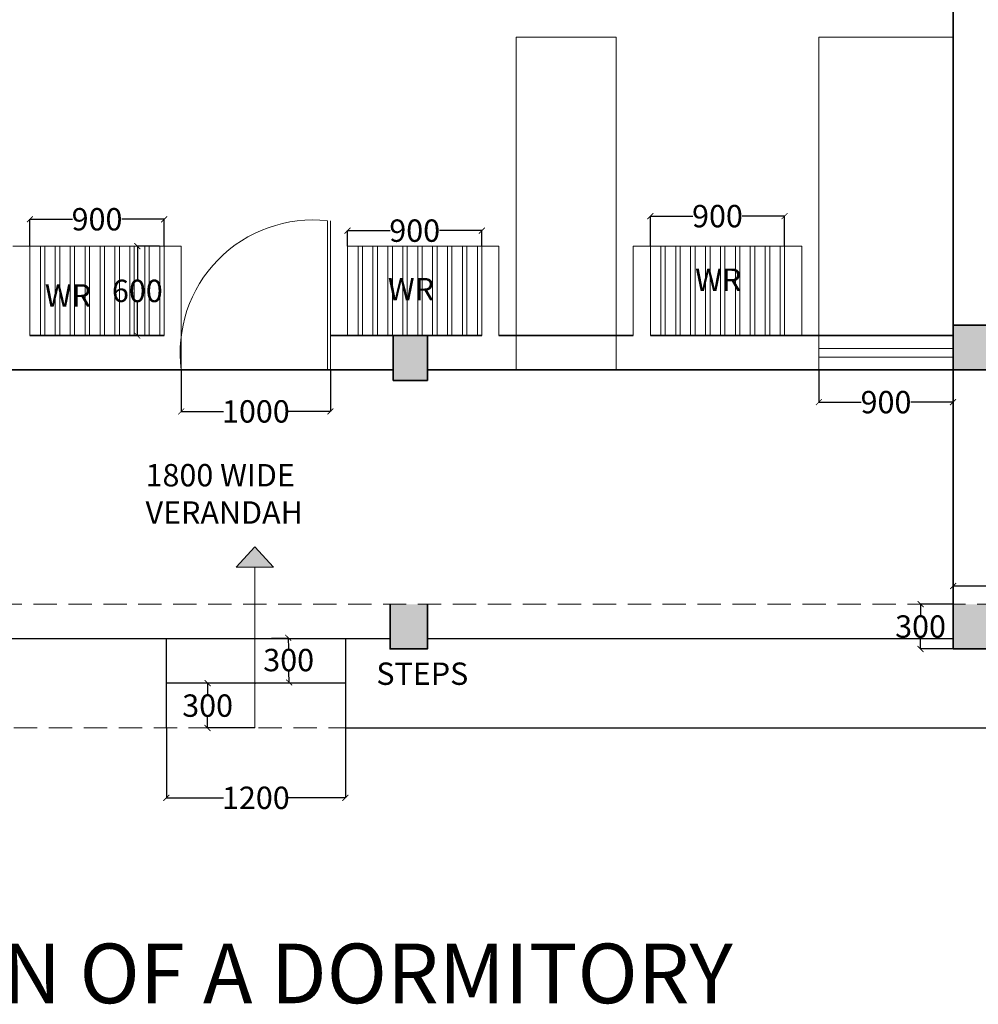
# Model space of a CAD drawing. Units: millimetres. Extents: x 32888 to 53184, y 27889 to 39696.
# Tile 4 of 6: x 41170 to 47598, y 27889 to 34489. Entities that reach past the tile are written whole.
import ezdxf

# ---------------------------------------------------------------- set-up
doc = ezdxf.new("R2010")
doc.units = ezdxf.units.MM
doc.header["$LTSCALE"] = 50
doc.header["$MEASUREMENT"] = 0
doc.linetypes.add('HIDDEN2', pattern=[0.1875, 0.125, -0.0625])
for name, color, linetype, lineweight in [('A-ANNO-DIMS', 2, 'Continuous', 18), ('A-ANNO-SYMB', 7, 'Continuous', 18), ('A-ANNO-SYMB-PATT', 18, 'Continuous', 13), ('A-ANNO-TEXT', 7, 'Continuous', 18), ('A-ANNO-TTLB', 152, 'Continuous', 35), ('A-AREA-IDEN', 7, 'Continuous', 18), ('A-COLS', 1, 'Continuous', 35), ('A-COLS-PATT', 18, 'Continuous', 18), ('A-DOOR', 4, 'Continuous', 18), ('A-FLOR-STRS', 7, 'Continuous', 25), ('A-FURN', 8, 'Continuous', 18), ('A-FURN-CASE', 8, 'Continuous', 18), ('A-GLAZ', 4, 'Continuous', 18), ('A-ROOF-OVHD', 8, 'HIDDEN2', 18), ('A-WALL', 7, 'Continuous', 35), ('A-WALL-HIDN', 7, 'HIDDEN2', 18), ('A-WALL-LOW', 7, 'Continuous', 25)]:
    doc.layers.add(name, color=color, linetype=linetype, lineweight=lineweight)
doc.styles.get("Standard").update_dxf_attribs({"font": 'arial.ttf'})
doc.dimstyles.get("Standard").update_dxf_attribs({"dimtxt": 150, "dimasz": 40, "dimexe": 0.18, "dimexo": 0.0625, "dimgap": 0.09, "dimtad": 0, "dimtih": 1, "dimtoh": 1, "dimdec": 0, "dimzin": 0, "dimdsep": 46, "dimtxsty": 'Standard', "dimblk": 'ARCHTICK', "dimcen": 0, "dimadec": 0, "dimazin": 0, "dimtfac": 1, "dimtdec": 0, "dimtofl": 0, "dimtmove": 0, "dimatfit": 3, "dimldrblk": 'ARCHTICK', "dimfxl": 1, "dimtolj": 1, "dimtzin": 0, "dimarcsym": 1})

# ---------------------------------------------------------------- blocks, each defined once
blk = doc.blocks.new('_ArchTick')
at = {"color": 0, "linetype": 'ByBlock', "const_width": 0.15}
blk.add_lwpolyline([(-0.5, -0.5), (0.5, 0.5)], dxfattribs=at)
blk = doc.blocks.new('*D1')
at = {"layer": 'A-ANNO-DIMS', "color": 0, "lineweight": -2, "ltscale": 50, "transparency": 16777216}
for p, q in [((42153.9, 29740.9), (42153.9, 29272.6)), ((43353.9, 29740.9), (43353.9, 29272.6)), ((42153.9, 29272.8), (42537.2, 29272.8)), ((43353.9, 29272.8), (42970.7, 29272.8))]:
    blk.add_line(p, q, dxfattribs=at)
at = {"layer": 'Defpoints', "color": 0, "ltscale": 50, "transparency": 16777216}
for p in [(42153.9, 29741), (43353.9, 29741), (43353.9, 29272.8)]:
    blk.add_point(p, dxfattribs=at)
at = {"layer": 'A-ANNO-DIMS', "color": 0, "lineweight": -2, "ltscale": 50, "transparency": 16777216, "xscale": 40, "yscale": 40, "zscale": 40, "rotation": 180}
blk.add_blockref('_ArchTick', (42153.9, 29272.8), dxfattribs=at)
at = {"layer": 'A-ANNO-DIMS', "color": 0, "lineweight": -2, "ltscale": 50, "transparency": 16777216, "xscale": 40, "yscale": 40, "zscale": 40}
blk.add_blockref('_ArchTick', (43353.9, 29272.8), dxfattribs=at)
at = {"layer": 'A-ANNO-DIMS', "color": 0, "ltscale": 50, "transparency": 16777216, "insert": (42753.9, 29272.8), "char_height": 150, "attachment_point": 5}
blk.add_mtext('\\A1;1200', dxfattribs=at)
blk = doc.blocks.new('*D3')
at = {"layer": 'A-ANNO-DIMS', "color": 0, "lineweight": -2, "ltscale": 50, "transparency": 16777216}
for p, q in [((42746.9, 30041), (42430.2, 30041)), ((42430.4, 30041), (42430.4, 29967.7)), ((42430.4, 29741), (42430.4, 29814.3)), ((42746.9, 29741), (42430.2, 29741))]:
    blk.add_line(p, q, dxfattribs=at)
at = {"layer": 'Defpoints', "color": 0, "ltscale": 50, "transparency": 16777216}
for p in [(42747, 30041), (42430.4, 29741), (42747, 29741)]:
    blk.add_point(p, dxfattribs=at)
at = {"layer": 'A-ANNO-DIMS', "color": 0, "lineweight": -2, "ltscale": 50, "transparency": 16777216, "xscale": 40, "yscale": 40, "zscale": 40}
for p, rotation in [((42430.4, 30041), 90), ((42430.4, 29741), 270)]:
    blk.add_blockref('_ArchTick', p, dxfattribs=dict(at, rotation=rotation))
at = {"layer": 'A-ANNO-DIMS', "color": 0, "ltscale": 50, "transparency": 16777216, "insert": (42430.4, 29891), "char_height": 150, "attachment_point": 5}
blk.add_mtext('\\A1;300', dxfattribs=at)
blk = doc.blocks.new('*D4')
at = {"layer": 'A-ANNO-DIMS', "color": 0, "lineweight": -2, "ltscale": 50, "transparency": 16777216}
for p, q in [((42747, 30341), (42970.6, 30346.2)), ((42970.4, 30346.2), (42972.1, 30272.9)), ((42977.4, 30046.2), (42975.7, 30119.5)), ((42754, 30041), (42977.6, 30046.2))]:
    blk.add_line(p, q, dxfattribs=at)
at = {"layer": 'Defpoints', "color": 0, "ltscale": 50, "transparency": 16777216}
for p in [(42747, 30341), (42970.4, 30346.2), (42753.9, 30041)]:
    blk.add_point(p, dxfattribs=at)
at = {"layer": 'A-ANNO-DIMS', "color": 0, "lineweight": -2, "ltscale": 50, "transparency": 16777216, "xscale": 40, "yscale": 40, "zscale": 40}
for p, rotation in [((42970.4, 30346.2), 91.33355342739812), ((42977.4, 30046.2), 271.3335534273981)]:
    blk.add_blockref('_ArchTick', p, dxfattribs=dict(at, rotation=rotation))
at = {"layer": 'A-ANNO-DIMS', "color": 0, "ltscale": 50, "transparency": 16777216, "insert": (42973.9, 30196.2), "char_height": 150, "attachment_point": 5}
blk.add_mtext('\\A1;300', dxfattribs=at)
blk = doc.blocks.new('*D8')
at = {"layer": 'A-ANNO-DIMS', "color": 0, "lineweight": -2, "ltscale": 50, "transparency": 16777216}
for p, q in [((47428.9, 30571.1), (47428.9, 30693)), ((47428.9, 30692.8), (47678.9, 30692.8)), ((47678.9, 30571.1), (47678.9, 30693)), ((47678.9, 30692.8), (47718.9, 30692.8))]:
    blk.add_line(p, q, dxfattribs=at)
at = {"layer": 'Defpoints', "color": 0, "ltscale": 50, "transparency": 16777216}
for p in [(47678.9, 30692.8), (47428.9, 30571), (47678.9, 30571)]:
    blk.add_point(p, dxfattribs=at)
at = {"layer": 'A-ANNO-DIMS', "color": 0, "lineweight": -2, "ltscale": 50, "transparency": 16777216, "xscale": 40, "yscale": 40, "zscale": 40, "rotation": 180}
blk.add_blockref('_ArchTick', (47428.9, 30692.8), dxfattribs=at)
at = {"layer": 'A-ANNO-DIMS', "color": 0, "lineweight": -2, "ltscale": 50, "transparency": 16777216, "xscale": 40, "yscale": 40, "zscale": 40}
blk.add_blockref('_ArchTick', (47678.9, 30692.8), dxfattribs=at)
at = {"layer": 'A-ANNO-DIMS', "color": 0, "ltscale": 50, "transparency": 16777216, "insert": (47885.8, 30692.8), "char_height": 150, "attachment_point": 5}
blk.add_mtext('\\A1;250', dxfattribs=at)
blk = doc.blocks.new('*D9')
at = {"layer": 'A-ANNO-DIMS', "color": 0, "lineweight": -2, "ltscale": 50, "transparency": 16777216}
for p, q in [((47428.9, 30571), (47210.4, 30571)), ((47210.6, 30571), (47210.6, 30497.7)), ((47210.6, 30271), (47210.6, 30344.3)), ((47428.9, 30271), (47210.4, 30271))]:
    blk.add_line(p, q, dxfattribs=at)
at = {"layer": 'Defpoints', "color": 0, "ltscale": 50, "transparency": 16777216}
for p in [(47210.6, 30571), (47428.9, 30571), (47428.9, 30271)]:
    blk.add_point(p, dxfattribs=at)
at = {"layer": 'A-ANNO-DIMS', "color": 0, "lineweight": -2, "ltscale": 50, "transparency": 16777216, "xscale": 40, "yscale": 40, "zscale": 40}
for p, rotation in [((47210.6, 30571), 90), ((47210.6, 30271), 270)]:
    blk.add_blockref('_ArchTick', p, dxfattribs=dict(at, rotation=rotation))
at = {"layer": 'A-ANNO-DIMS', "color": 0, "ltscale": 50, "transparency": 16777216, "insert": (47210.6, 30421), "char_height": 150, "attachment_point": 5}
blk.add_mtext('\\A1;300', dxfattribs=at)
blk = doc.blocks.new('*D12')
at = {"layer": 'A-ANNO-DIMS', "color": 0, "lineweight": -2, "ltscale": 50, "transparency": 16777216}
for p, q in [((43368.9, 32971.1), (43368.9, 33075.2)), ((43368.9, 33075), (43653.4, 33075)), ((44268.9, 33075), (43984.5, 33075)), ((44268.9, 32971.1), (44268.9, 33075.2))]:
    blk.add_line(p, q, dxfattribs=at)
at = {"layer": 'Defpoints', "color": 0, "ltscale": 50, "transparency": 16777216}
for p in [(43368.9, 33075), (43368.9, 32971), (44268.9, 32971)]:
    blk.add_point(p, dxfattribs=at)
at = {"layer": 'A-ANNO-DIMS', "color": 0, "lineweight": -2, "ltscale": 50, "transparency": 16777216, "xscale": 40, "yscale": 40, "zscale": 40, "rotation": 180}
blk.add_blockref('_ArchTick', (43368.9, 33075), dxfattribs=at)
at = {"layer": 'A-ANNO-DIMS', "color": 0, "lineweight": -2, "ltscale": 50, "transparency": 16777216, "xscale": 40, "yscale": 40, "zscale": 40}
blk.add_blockref('_ArchTick', (44268.9, 33075), dxfattribs=at)
at = {"layer": 'A-ANNO-DIMS', "color": 0, "ltscale": 50, "transparency": 16777216, "insert": (43818.9, 33075), "char_height": 150, "attachment_point": 5}
blk.add_mtext('\\A1;900', dxfattribs=at)
blk = doc.blocks.new('*D13')
at = {"layer": 'A-ANNO-DIMS', "color": 0, "lineweight": -2, "ltscale": 50, "transparency": 16777216}
for p, q in [((41238.9, 32971.1), (41238.9, 33151.5)), ((41238.9, 33151.3), (41523.4, 33151.3)), ((42138.9, 33151.3), (41854.5, 33151.3)), ((42138.9, 32971.1), (42138.9, 33151.5))]:
    blk.add_line(p, q, dxfattribs=at)
at = {"layer": 'Defpoints', "color": 0, "ltscale": 50, "transparency": 16777216}
for p in [(41238.9, 33151.3), (41238.9, 32971), (42138.9, 32971)]:
    blk.add_point(p, dxfattribs=at)
at = {"layer": 'A-ANNO-DIMS', "color": 0, "lineweight": -2, "ltscale": 50, "transparency": 16777216, "xscale": 40, "yscale": 40, "zscale": 40}
for p, rotation in [((41238.9, 33151.3), 179.9999999999991), ((42138.9, 33151.3), 359.9999999999991)]:
    blk.add_blockref('_ArchTick', p, dxfattribs=dict(at, rotation=rotation))
at = {"layer": 'A-ANNO-DIMS', "color": 0, "ltscale": 50, "transparency": 16777216, "insert": (41688.9, 33151.3), "char_height": 150, "attachment_point": 5}
blk.add_mtext('\\A1;900', dxfattribs=at)
blk = doc.blocks.new('*D17')
at = {"layer": 'A-ANNO-DIMS', "color": 0, "lineweight": -2, "ltscale": 50, "transparency": 16777216}
for p, q in [((42253.9, 32140.9), (42253.9, 31863)), ((43253.9, 32140.9), (43253.9, 31863)), ((42253.9, 31863.2), (42537.2, 31863.2)), ((43253.9, 31863.2), (42970.7, 31863.2))]:
    blk.add_line(p, q, dxfattribs=at)
at = {"layer": 'Defpoints', "color": 0, "ltscale": 50, "transparency": 16777216}
for p in [(42253.9, 32141), (43253.9, 32141), (43253.9, 31863.2)]:
    blk.add_point(p, dxfattribs=at)
at = {"layer": 'A-ANNO-DIMS', "color": 0, "lineweight": -2, "ltscale": 50, "transparency": 16777216, "xscale": 40, "yscale": 40, "zscale": 40, "rotation": 180}
blk.add_blockref('_ArchTick', (42253.9, 31863.2), dxfattribs=at)
at = {"layer": 'A-ANNO-DIMS', "color": 0, "lineweight": -2, "ltscale": 50, "transparency": 16777216, "xscale": 40, "yscale": 40, "zscale": 40}
blk.add_blockref('_ArchTick', (43253.9, 31863.2), dxfattribs=at)
at = {"layer": 'A-ANNO-DIMS', "color": 0, "ltscale": 50, "transparency": 16777216, "insert": (42753.9, 31863.2), "char_height": 150, "attachment_point": 5}
blk.add_mtext('\\A1;1000', dxfattribs=at)
blk = doc.blocks.new('*D19')
at = {"layer": 'A-ANNO-DIMS', "color": 0, "lineweight": -2, "ltscale": 50, "transparency": 16777216}
for p, q in [((45398.9, 32971.1), (45398.9, 33172.5)), ((45398.9, 33172.3), (45683.4, 33172.3)), ((46298.9, 33172.3), (46014.5, 33172.3)), ((46298.9, 32971.1), (46298.9, 33172.5))]:
    blk.add_line(p, q, dxfattribs=at)
at = {"layer": 'Defpoints', "color": 0, "ltscale": 50, "transparency": 16777216}
for p in [(46298.9, 33172.3), (45398.9, 32971), (46298.9, 32971)]:
    blk.add_point(p, dxfattribs=at)
at = {"layer": 'A-ANNO-DIMS', "color": 0, "lineweight": -2, "ltscale": 50, "transparency": 16777216, "xscale": 40, "yscale": 40, "zscale": 40, "rotation": 180}
blk.add_blockref('_ArchTick', (45398.9, 33172.3), dxfattribs=at)
at = {"layer": 'A-ANNO-DIMS', "color": 0, "lineweight": -2, "ltscale": 50, "transparency": 16777216, "xscale": 40, "yscale": 40, "zscale": 40}
blk.add_blockref('_ArchTick', (46298.9, 33172.3), dxfattribs=at)
at = {"layer": 'A-ANNO-DIMS', "color": 0, "ltscale": 50, "transparency": 16777216, "insert": (45848.9, 33172.3), "char_height": 150, "attachment_point": 5}
blk.add_mtext('\\A1;900', dxfattribs=at)
blk = doc.blocks.new('*D20')
at = {"layer": 'A-ANNO-DIMS', "color": 0, "lineweight": -2, "ltscale": 50, "transparency": 16777216}
for p, q in [((42108.9, 32971), (41959.2, 32971)), ((41959.3, 32971), (41959.3, 32747.7)), ((41959.3, 32371), (41959.3, 32594.3)), ((42108.9, 32371), (41959.2, 32371))]:
    blk.add_line(p, q, dxfattribs=at)
at = {"layer": 'Defpoints', "color": 0, "ltscale": 50, "transparency": 16777216}
for p in [(41959.3, 32971), (42108.9, 32971), (42108.9, 32371)]:
    blk.add_point(p, dxfattribs=at)
at = {"layer": 'A-ANNO-DIMS', "color": 0, "lineweight": -2, "ltscale": 50, "transparency": 16777216, "xscale": 40, "yscale": 40, "zscale": 40}
for p, rotation in [((41959.3, 32971), 90), ((41959.3, 32371), 270)]:
    blk.add_blockref('_ArchTick', p, dxfattribs=dict(at, rotation=rotation))
at = {"layer": 'A-ANNO-DIMS', "color": 0, "ltscale": 50, "transparency": 16777216, "insert": (41959.3, 32671), "char_height": 150, "attachment_point": 5}
blk.add_mtext('\\A1;600', dxfattribs=at)
blk = doc.blocks.new('*D21')
at = {"layer": 'A-ANNO-DIMS', "color": 0, "lineweight": -2, "ltscale": 50, "transparency": 16777216}
for p, q in [((46528.9, 32140.9), (46528.9, 31925.1)), ((47428.9, 32140.9), (47428.9, 31925.1)), ((46528.9, 31925.3), (46813.4, 31925.3)), ((47428.9, 31925.3), (47144.5, 31925.3))]:
    blk.add_line(p, q, dxfattribs=at)
at = {"layer": 'Defpoints', "color": 0, "ltscale": 50, "transparency": 16777216}
for p in [(46528.9, 32141), (47428.9, 32141), (46528.9, 31925.3)]:
    blk.add_point(p, dxfattribs=at)
at = {"layer": 'A-ANNO-DIMS', "color": 0, "lineweight": -2, "ltscale": 50, "transparency": 16777216, "xscale": 40, "yscale": 40, "zscale": 40, "rotation": 180}
blk.add_blockref('_ArchTick', (46528.9, 31925.3), dxfattribs=at)
at = {"layer": 'A-ANNO-DIMS', "color": 0, "lineweight": -2, "ltscale": 50, "transparency": 16777216, "xscale": 40, "yscale": 40, "zscale": 40}
blk.add_blockref('_ArchTick', (47428.9, 31925.3), dxfattribs=at)
at = {"layer": 'A-ANNO-DIMS', "color": 0, "ltscale": 50, "transparency": 16777216, "insert": (46978.9, 31925.3), "char_height": 150, "attachment_point": 5}
blk.add_mtext('\\A1;900', dxfattribs=at)
blk = doc.blocks.new('BED-SINGLE-900')
for p in [(900, 2230), (0, 0)]:
    blk.add_line(p, (900, 0))
blk = doc.blocks.new('BED-NARROW-670')
for p, q in [((0, 2230), (0, 0)), ((670, 2230), (670, 0)), ((0, 0), (670, 0))]:
    blk.add_line(p, q)
blk = doc.blocks.new('WARDROBE-SLATTED-PANEL-900')
at = {"ltscale": 50}
for p, q in [((-830, 600), (-830, 0)), ((-800, 600), (-800, 0)), ((-730, 600), (-730, 0)), ((-700, 600), (-700, 0)), ((-630, 600), (-630, 0)), ((-600, 600), (-600, 0)), ((-530, 600), (-530, 0)), ((-500, 600), (-500, 0)), ((-430, 600), (-430, 0)), ((-400, 600), (-400, 0)), ((-330, 600), (-330, 0)), ((-300, 600), (-300, 0)), ((-230, 600), (-230, 0)), ((-200, 600), (-200, 0)), ((-130, 600), (-130, 0)), ((-100, 600), (-100, 0)), ((-30, 600), (-30, 0)), ((-30, 0), (0, 0))]:
    blk.add_line(p, q, dxfattribs=at)
blk = doc.blocks.new('DOOR-SINGLE-1000')
at = {"ltscale": 50}
for p, q in [((987.6, 0), (987.6, 1000)), ((1007.6, 0), (1007.6, 1000))]:
    blk.add_line(p, q, dxfattribs=at)
blk.add_arc((889, 116.4), 889, 83.63161, 187.52584, dxfattribs=at)
blk = doc.blocks.new('WINDOW-900')
for p, q in [((900, 60), (0, 60)), ((900, 0), (0, 0))]:
    blk.add_line(p, q)
blk = doc.blocks.new('COLUMN-EDGE-230x300')
for points in [[(0, 300), (0, 0)], [(230, 0), (230, 300)], [(230, 0), (0, 0)]]:
    blk.add_lwpolyline(points)
blk = doc.blocks.new('COLUMN-VERANDAH-250x300')
blk.add_lwpolyline([(0, 300), (0, 0), (250, 0), (250, 300)])
blk = doc.blocks.new('*D77')
at = {"layer": 'A-ANNO-DIMS', "color": 0, "lineweight": -2, "ltscale": 50, "transparency": 16777216}
for p, q in [((50889, 38071), (52833.2, 38071)), ((52833, 38071), (52833, 33982.7)), ((52833, 29741), (52833, 33829.3)), ((43354, 29741), (52833.2, 29741))]:
    blk.add_line(p, q, dxfattribs=at)
at = {"layer": 'Defpoints', "color": 0, "ltscale": 50, "transparency": 16777216}
for p in [(50888.9, 38071), (43353.9, 29741), (52833, 29741)]:
    blk.add_point(p, dxfattribs=at)
at = {"layer": 'A-ANNO-DIMS', "color": 0, "lineweight": -2, "ltscale": 50, "transparency": 16777216, "xscale": 40, "yscale": 40, "zscale": 40}
for p, rotation in [((52833, 38071), 90), ((52833, 29741), 270)]:
    blk.add_blockref('_ArchTick', p, dxfattribs=dict(at, rotation=rotation))
at = {"layer": 'A-ANNO-DIMS', "color": 0, "ltscale": 50, "transparency": 16777216, "insert": (52833, 33906), "char_height": 150, "attachment_point": 5}
blk.add_mtext('\\A1;8330', dxfattribs=at)

msp = doc.modelspace()

# ---------------------------------------------------------------- hatches: boundary and pattern name
at = {"layer": 'A-ANNO-SYMB-PATT', "ltscale": 50}
h = msp.add_hatch(color=256, dxfattribs=at)
h.dxf.hatch_style = 1
h.paths.add_polyline_path([(42746.97, 30954.79), (42621.34, 30818.07), (42746.97, 30818.07), (42872.59, 30818.07)])
at = {"layer": 'A-COLS-PATT', "ltscale": 50}
h = msp.add_hatch(color=256, dxfattribs=at)
h.dxf.hatch_style = 1
h.paths.add_polyline_path([(35398.95, 38071.01), (35168.95, 38071.01), (35168.95, 37771.01), (35398.95, 37771.01)])
h.paths.add_polyline_path([(39628.95, 38071.01), (39398.95, 38071.01), (39398.95, 37771.01), (39628.95, 37771.01)])
h.paths.add_polyline_path([(43903.95, 38071.01), (43673.95, 38071.01), (43673.95, 37771.01), (43903.95, 37771.01)])
h.paths.add_polyline_path([(47658.95, 38071.01), (47428.95, 38071.01), (47428.95, 37771.01), (47658.95, 37771.01)])
h.paths.add_polyline_path([(50888.95, 38071.01), (50658.95, 38071.01), (50658.95, 37771.01), (50888.95, 37771.01)])
h.paths.add_polyline_path([(50888.95, 35221.01), (50658.95, 35221.01), (50658.95, 34921.01), (50888.95, 34921.01)])
h.paths.add_polyline_path([(47658.95, 35221.01), (47428.95, 35221.01), (47428.95, 34921.01), (47658.95, 34921.01)])
h.paths.add_polyline_path([(39628.95, 35071.01), (39628.95, 35221.01), (39398.95, 35221.01), (39398.95, 34921.01), (39628.95, 34921.01)])
h.paths.add_polyline_path([(35398.95, 35221.01), (35168.95, 35221.01), (35168.95, 34921.01), (35398.95, 34921.01)])
h.paths.add_polyline_path([(35398.95, 32371.01), (35168.95, 32371.01), (35168.95, 32071.01), (35398.95, 32071.01)])
h.paths.add_polyline_path([(35418.95, 30571.01), (35168.95, 30571.01), (35168.95, 30271.01), (35418.95, 30271.01)])
h.paths.add_polyline_path([(39642.61, 30571.01), (39392.61, 30571.01), (39392.61, 30271.01), (39642.61, 30271.01)])
h.paths.add_polyline_path([(39628.95, 32371.01), (39398.95, 32371.01), (39398.95, 32071.01), (39628.95, 32071.01)])
h.paths.add_polyline_path([(43903.95, 32371.01), (43673.95, 32371.01), (43673.95, 32071.01), (43903.95, 32071.01)])
h.paths.add_polyline_path([(43903.95, 30571.01), (43653.95, 30571.01), (43653.95, 30271.01), (43903.95, 30271.01)])
h.paths.add_polyline_path([(47658.95, 32441.01), (47428.95, 32441.01), (47428.95, 32141.01), (47658.95, 32141.01)])
h.paths.add_polyline_path([(50888.95, 32414.45), (50658.95, 32414.45), (50658.95, 32114.45), (50888.95, 32114.45)])
h.paths.add_polyline_path([(50888.95, 30571.01), (50638.95, 30571.01), (50638.95, 30271.01), (50888.95, 30271.01)])
h.paths.add_polyline_path([(47678.95, 30571.01), (47428.95, 30571.01), (47428.95, 30341.01), (47678.95, 30341.01)])
h.paths.add_polyline_path([(47678.95, 30341.01), (47428.95, 30341.01), (47428.95, 30271.01), (47678.95, 30271.01)])

# ---------------------------------------------------------------- linework, layer by layer
at = {"layer": 'A-ANNO-SYMB', "ltscale": 50}
for p, q in [((42746.97, 30954.79), (42621.34, 30818.07)), ((42746.97, 30954.79), (42872.59, 30818.07)), ((42621.34, 30818.07), (42746.97, 30818.07)), ((42746.97, 29741.01), (42746.97, 30818.07)), ((42872.59, 30818.07), (42746.97, 30818.07))]:
    msp.add_line(p, q, dxfattribs=at)
at = {"layer": 'A-COLS'}
for points in [[(47658.95, 32441.01), (47428.95, 32441.01)], [(47428.95, 30271.01), (47678.95, 30271.01), (47678.95, 30571.01)]]:
    msp.add_lwpolyline(points, dxfattribs=at)
at = {"layer": 'A-FLOR-STRS', "ltscale": 50}
for p, q in [((42153.95, 29741.01), (42153.95, 30341.01)), ((43353.95, 30341.01), (43353.95, 29741.01)), ((43353.95, 30041.01), (42153.95, 30041.01))]:
    msp.add_line(p, q, dxfattribs=at)
at = {"layer": 'A-FURN-CASE'}
for p, q in [((42253.95, 32971.01), (41123.95, 32971.01)), ((41238.95, 32371.01), (41238.95, 32971.01)), ((42138.95, 32971.01), (42138.95, 32371.01)), ((42253.95, 32141.01), (42253.95, 32971.01)), ((43253.95, 32141.01), (43253.95, 32971.01)), ((43368.95, 32371.01), (43368.95, 32971.01)), ((44383.95, 32971.01), (43368.95, 32971.01)), ((44268.95, 32371.01), (44268.95, 32971.01)), ((44383.95, 32371.01), (44383.95, 32971.01)), ((45398.95, 32971.01), (45283.95, 32971.01)), ((45283.95, 32971.01), (45283.95, 32371.01)), ((45398.95, 32371.01), (45398.95, 32971.01)), ((46413.95, 32971.01), (46298.95, 32971.01)), ((46298.95, 32971.01), (46298.95, 32371.01)), ((46413.95, 32371.01), (46413.95, 32971.01))]:
    msp.add_line(p, q, dxfattribs=at)
at = {"layer": 'A-FURN-CASE', "ltscale": 50}
msp.add_line((45398.95, 32971.01), (46298.95, 32971.01), dxfattribs=at)
at = {"layer": 'A-ROOF-OVHD', "ltscale": 25}
msp.add_line((34568.95, 29741.01), (51488.95, 29741.01), dxfattribs=at)
at = {"layer": 'A-WALL'}
for p, q in [((47428.95, 38071.01), (47428.95, 30271.01)), ((41238.95, 32371.01), (42138.95, 32371.01)), ((43253.95, 32371.01), (44268.95, 32371.01)), ((44383.95, 32371.01), (45283.95, 32371.01)), ((45398.95, 32371.01), (47428.95, 32371.01)), ((39628.95, 32141.01), (43673.95, 32141.01)), ((43903.95, 32141.01), (47658.95, 32141.01))]:
    msp.add_line(p, q, dxfattribs=at)
at = {"layer": 'A-WALL-HIDN', "ltscale": 25}
msp.add_line((35168.95, 30571.01), (50888.95, 30571.01), dxfattribs=at)
at = {"layer": 'A-WALL-LOW'}
for p, q in [((39642.61, 30341.01), (43653.95, 30341.01)), ((43903.95, 30341.01), (47428.95, 30341.01))]:
    msp.add_line(p, q, dxfattribs=at)

# ---------------------------------------------------------------- block references
at = {"layer": 'A-COLS'}
for name, p in [('COLUMN-EDGE-230x300', (43673.95, 32071.01)), ('COLUMN-VERANDAH-250x300', (43653.95, 30271.01))]:
    msp.add_blockref(name, p, dxfattribs=at)
at = {"layer": 'A-DOOR'}
msp.add_blockref('DOOR-SINGLE-1000', (42246.34, 32141.01), dxfattribs=at)
at = {"layer": 'A-FURN', "rotation": 180}
for name, p in [('BED-NARROW-670', (45168.95, 34371.01)), ('BED-SINGLE-900', (47428.95, 34371.01))]:
    msp.add_blockref(name, p, dxfattribs=at)
at = {"layer": 'A-FURN-CASE'}
for p in [(42138.95, 32371.01), (44268.95, 32371.01), (46298.95, 32371.01)]:
    msp.add_blockref('WARDROBE-SLATTED-PANEL-900', p, dxfattribs=at)
at = {"layer": 'A-GLAZ'}
msp.add_blockref('WINDOW-900', (46528.95, 32226.01), dxfattribs=at)

# ---------------------------------------------------------------- texts
at = {"layer": 'A-ANNO-TEXT', "ltscale": 50, "char_height": 150, "attachment_point": 1}
for s, width, insert in [('WR', 742.516, (45698.95, 32821.01)), ('WR', 742.516, (43638.95, 32758.02)), ('WR', 742.516, (41338.95, 32715.79)), ('STEPS', 901.3249, (43561.71, 30179.87))]:
    msp.add_mtext_dynamic_manual_height_columns(s, width=width, gutter_width=1, heights=[0], dxfattribs=dict(at, insert=insert))
at = {"layer": 'A-ANNO-TTLB', "ltscale": 50, "insert": (40080.77, 28295.74), "char_height": 400, "attachment_point": 1}
msp.add_mtext_dynamic_manual_height_columns('PLAN OF A DORMITORY', width=8577.7498, gutter_width=1, heights=[0], dxfattribs=at)
at = {"layer": 'A-AREA-IDEN', "ltscale": 50, "insert": (42014.21, 31510.44), "char_height": 150, "attachment_point": 1}
msp.add_mtext_dynamic_manual_height_columns('1800 WIDE\\PVERANDAH', width=2041.7469, gutter_width=1, heights=[0], dxfattribs=at)

# ---------------------------------------------------------------- dimensions: what is measured, and where the dimension line sits
at = {"layer": 'A-ANNO-DIMS', "ltscale": 50}
dim = msp.add_linear_dim(base=(52833.03, 29741.01), p1=(50888.95, 38071.01), p2=(43353.95, 29741.01), angle=90, dimstyle='Standard', override={"dimdec": 0, "dimlfac": 1, "dimrnd": 0, "dimzin": 0, "dimdsep": 46, "dimlunit": 2}, dxfattribs=at)
dim.commit()
dim.dimension.update_dxf_attribs({"geometry": '*D77', "text_midpoint": (52833.03, 33906.01)})
for p1, p2, distance, picture, middle in [((45398.95, 32971.01), (46298.95, 32971.01), 201.31, '*D19', (45848.95, 33172.32)), ((42138.95, 32971.01), (41238.95, 32971.01), -180.33, '*D13', (41688.95, 33151.34)), ((44268.95, 32971.01), (43368.95, 32971.01), -104.03, '*D12', (43818.95, 33075.04)), ((42108.95, 32371.01), (42108.95, 32971.01), 149.61, '*D20', (41959.34, 32671.01)), ((42253.95, 32141.01), (43253.95, 32141.01), -277.8, '*D17', (42753.95, 31863.21)), ((47428.95, 32141.01), (46528.95, 32141.01), 215.73, '*D21', (46978.95, 31925.28)), ((47428.95, 30571.01), (47678.95, 30571.01), 121.77, '*D8', (47885.77, 30692.78)), ((47428.95, 30271.01), (47428.95, 30571.01), 218.36, '*D9', (47210.59, 30421.01)), ((42753.95, 30041.01), (42746.97, 30341.01), -223.51, '*D4', (42973.91, 30196.21)), ((42746.97, 30041.01), (42746.97, 29741.01), -316.55, '*D3', (42430.42, 29891.01))]:
    dim = msp.add_aligned_dim(p1=p1, p2=p2, distance=distance, dimstyle='Standard', override={"dimclrd": 0, "dimclre": 0, "dimclrt": 0}, dxfattribs=at)
    dim.commit()
    dim.dimension.update_dxf_attribs({"geometry": picture, "text_midpoint": middle})
dim = msp.add_linear_dim(base=(43353.95, 29272.8), p1=(42153.95, 29741.01), p2=(43353.95, 29741.01), dimstyle='Standard', override={"dimclrd": 0, "dimclre": 0, "dimclrt": 0}, dxfattribs=at)
dim.commit()
dim.dimension.update_dxf_attribs({"geometry": '*D1', "text_midpoint": (42753.95, 29272.8)})

doc.saveas('drawing.dxf')
